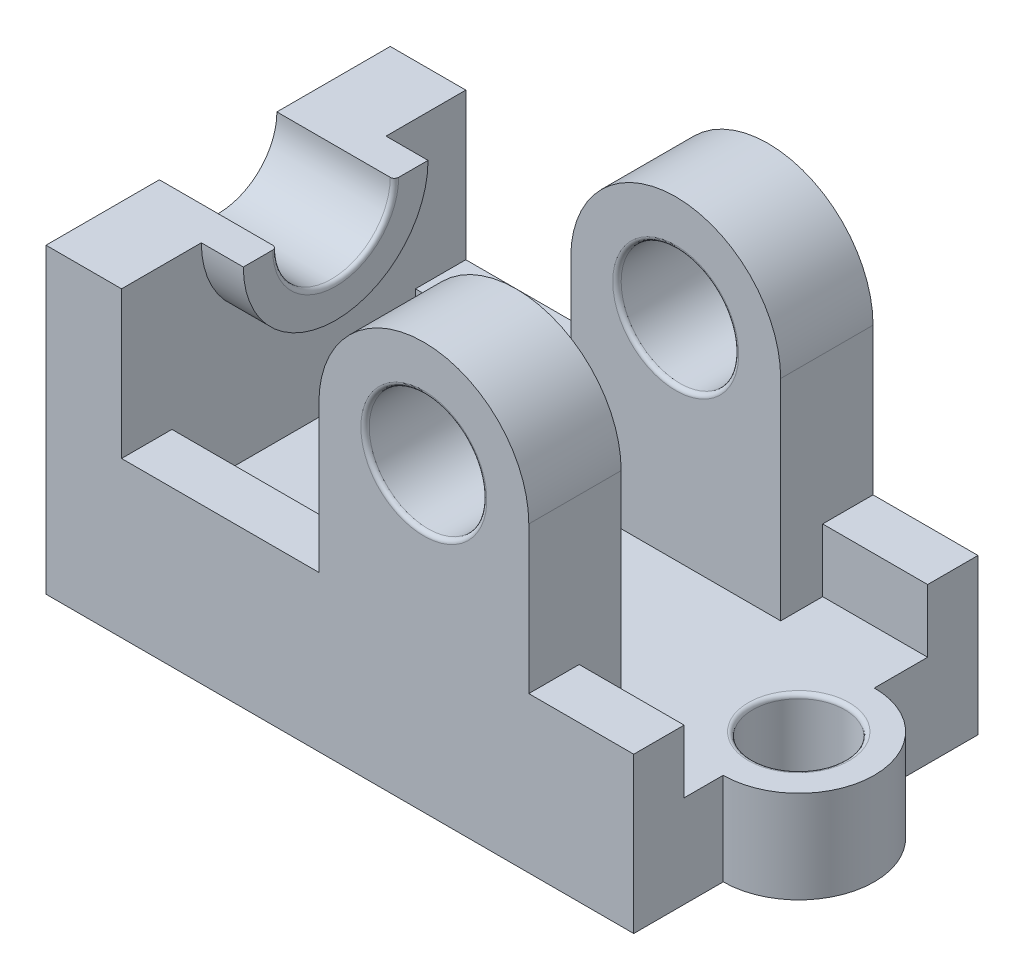
ISO-10303-21;
HEADER;
FILE_DESCRIPTION(('STEP AP214'),'2;1');
FILE_NAME('part.step','',(''),(''),'','','');
FILE_SCHEMA(('AUTOMOTIVE_DESIGN { 1 0 10303 214 1 1 1 1 }'));
ENDSEC;
DATA;
#1=APPLICATION_CONTEXT('core data for automotive mechanical design processes');
#2=APPLICATION_PROTOCOL_DEFINITION('international standard','automotive_design',2000,#1);
#3=PRODUCT_CONTEXT('',#1,'mechanical');
#4=PRODUCT('Part','Part','',(#3));
#5=PRODUCT_RELATED_PRODUCT_CATEGORY('part','',(#4));
#6=PRODUCT_DEFINITION_FORMATION('','',#4);
#7=PRODUCT_DEFINITION_CONTEXT('part definition',#1,'design');
#8=PRODUCT_DEFINITION('design','',#6,#7);
#9=PRODUCT_DEFINITION_SHAPE('','',#8);
#10=(LENGTH_UNIT() NAMED_UNIT(*) SI_UNIT(.MILLI.,.METRE.));
#11=(NAMED_UNIT(*) PLANE_ANGLE_UNIT() SI_UNIT($,.RADIAN.));
#12=(NAMED_UNIT(*) SI_UNIT($,.STERADIAN.) SOLID_ANGLE_UNIT());
#13=UNCERTAINTY_MEASURE_WITH_UNIT(LENGTH_MEASURE(1.E-05),#10,'distance_accuracy_value','');
#14=(GEOMETRIC_REPRESENTATION_CONTEXT(3) GLOBAL_UNCERTAINTY_ASSIGNED_CONTEXT((#13)) GLOBAL_UNIT_ASSIGNED_CONTEXT((#10,
#11,#12)) REPRESENTATION_CONTEXT('',''));
#15=CARTESIAN_POINT('',(0.,0.,0.));
#16=DIRECTION('',(0.,0.,1.));
#17=DIRECTION('',(1.,0.,0.));
#18=AXIS2_PLACEMENT_3D('',#15,#16,#17);
#19=CARTESIAN_POINT('',(0.,72.,0.));
#20=DIRECTION('',(0.,-1.,0.));
#21=DIRECTION('',(0.,0.,-1.));
#22=AXIS2_PLACEMENT_3D('',#19,#20,#21);
#23=PLANE('',#22);
#24=DIRECTION('',(0.,0.,1.));
#25=VECTOR('',#24,1.);
#26=CARTESIAN_POINT('',(-70.,72.,41.));
#27=LINE('',#26,#25);
#28=CARTESIAN_POINT('',(-70.,72.,-41.));
#29=VERTEX_POINT('',#28);
#30=CARTESIAN_POINT('',(-70.,72.,-14.));
#31=VERTEX_POINT('',#30);
#32=EDGE_CURVE('E270',#29,#31,#27,.T.);
#33=ORIENTED_EDGE('',*,*,#32,.T.);
#34=DIRECTION('',(-1.,0.,0.));
#35=VECTOR('',#34,1.);
#36=CARTESIAN_POINT('',(-42.,72.,-14.));
#37=LINE('',#36,#35);
#38=CARTESIAN_POINT('',(-43.,72.,-14.));
#39=VERTEX_POINT('',#38);
#40=EDGE_CURVE('E256',#39,#31,#37,.T.);
#41=ORIENTED_EDGE('',*,*,#40,.F.);
#42=CARTESIAN_POINT('',(-43.,72.,-15.));
#43=DIRECTION('',(0.,-1.,0.));
#44=DIRECTION('',(0.,0.,-1.));
#45=AXIS2_PLACEMENT_3D('',#42,#43,#44);
#46=CIRCLE('',#45,1.);
#47=CARTESIAN_POINT('',(-42.,72.,-15.));
#48=VERTEX_POINT('',#47);
#49=EDGE_CURVE('E63',#39,#48,#46,.F.);
#50=ORIENTED_EDGE('',*,*,#49,.T.);
#51=DIRECTION('',(0.,0.,-1.));
#52=VECTOR('',#51,1.);
#53=CARTESIAN_POINT('',(-42.,72.,-14.));
#54=LINE('',#53,#52);
#55=CARTESIAN_POINT('',(-42.,72.,-22.));
#56=VERTEX_POINT('',#55);
#57=EDGE_CURVE('E263',#48,#56,#54,.T.);
#58=ORIENTED_EDGE('',*,*,#57,.T.);
#59=DIRECTION('',(-1.,0.,0.));
#60=VECTOR('',#59,1.);
#61=CARTESIAN_POINT('',(-42.,72.,-22.));
#62=LINE('',#61,#60);
#63=CARTESIAN_POINT('',(-52.,72.,-22.));
#64=VERTEX_POINT('',#63);
#65=EDGE_CURVE('E544',#56,#64,#62,.T.);
#66=ORIENTED_EDGE('',*,*,#65,.T.);
#67=DIRECTION('',(0.,0.,-1.));
#68=VECTOR('',#67,1.);
#69=CARTESIAN_POINT('',(-52.,72.,-41.));
#70=LINE('',#69,#68);
#71=CARTESIAN_POINT('',(-52.,72.,-41.));
#72=VERTEX_POINT('',#71);
#73=EDGE_CURVE('E590',#64,#72,#70,.T.);
#74=ORIENTED_EDGE('',*,*,#73,.T.);
#75=DIRECTION('',(-1.,0.,0.));
#76=VECTOR('',#75,1.);
#77=CARTESIAN_POINT('',(-70.,72.,-41.));
#78=LINE('',#77,#76);
#79=EDGE_CURVE('E269',#72,#29,#78,.T.);
#80=ORIENTED_EDGE('',*,*,#79,.T.);
#81=EDGE_LOOP('',(#33,#41,#50,#58,#66,#74,#80));
#82=FACE_BOUND('',#81,.T.);
#83=ADVANCED_FACE('F47',(#82),#23,.F.);
#84=CARTESIAN_POINT('',(70.,22.,1.69184290030211));
#85=DIRECTION('',(0.,1.,0.));
#86=DIRECTION('',(0.,0.,1.));
#87=AXIS2_PLACEMENT_3D('',#84,#85,#86);
#88=PLANE('',#87);
#89=CARTESIAN_POINT('',(70.,22.,1.69184290030211));
#90=DIRECTION('',(0.,1.,0.));
#91=DIRECTION('',(0.,0.,1.));
#92=AXIS2_PLACEMENT_3D('',#89,#90,#91);
#93=CIRCLE('',#92,12.);
#94=CARTESIAN_POINT('',(70.,22.,13.6918429003021));
#95=VERTEX_POINT('',#94);
#96=EDGE_CURVE('E418',#95,#95,#93,.F.);
#97=ORIENTED_EDGE('',*,*,#96,.T.);
#98=EDGE_LOOP('',(#97));
#99=FACE_BOUND('',#98,.T.);
#100=DIRECTION('',(-1.,0.,0.));
#101=VECTOR('',#100,1.);
#102=CARTESIAN_POINT('',(0.,22.,-29.));
#103=LINE('',#102,#101);
#104=CARTESIAN_POINT('',(-4.99999999999997,22.,-29.));
#105=VERTEX_POINT('',#104);
#106=CARTESIAN_POINT('',(-52.,22.,-29.));
#107=VERTEX_POINT('',#106);
#108=EDGE_CURVE('E304',#105,#107,#103,.T.);
#109=ORIENTED_EDGE('',*,*,#108,.T.);
#110=DIRECTION('',(0.,0.,-1.));
#111=VECTOR('',#110,1.);
#112=CARTESIAN_POINT('',(-52.,22.,-41.));
#113=LINE('',#112,#111);
#114=CARTESIAN_POINT('',(-52.,22.,29.));
#115=VERTEX_POINT('',#114);
#116=EDGE_CURVE('E276',#115,#107,#113,.T.);
#117=ORIENTED_EDGE('',*,*,#116,.F.);
#118=DIRECTION('',(-1.,0.,0.));
#119=VECTOR('',#118,1.);
#120=CARTESIAN_POINT('',(0.,22.,29.));
#121=LINE('',#120,#119);
#122=CARTESIAN_POINT('',(-4.99999999999997,22.,29.));
#123=VERTEX_POINT('',#122);
#124=EDGE_CURVE('E328',#123,#115,#121,.T.);
#125=ORIENTED_EDGE('',*,*,#124,.F.);
#126=DIRECTION('',(0.,0.,1.));
#127=VECTOR('',#126,1.);
#128=CARTESIAN_POINT('',(-4.99999999999998,22.,19.));
#129=LINE('',#128,#127);
#130=CARTESIAN_POINT('',(-4.99999999999998,22.,19.));
#131=VERTEX_POINT('',#130);
#132=EDGE_CURVE('E577',#131,#123,#129,.T.);
#133=ORIENTED_EDGE('',*,*,#132,.F.);
#134=DIRECTION('',(-1.,0.,0.));
#135=VECTOR('',#134,1.);
#136=CARTESIAN_POINT('',(45.,22.,19.));
#137=LINE('',#136,#135);
#138=CARTESIAN_POINT('',(45.,22.,19.));
#139=VERTEX_POINT('',#138);
#140=EDGE_CURVE('E290',#139,#131,#137,.T.);
#141=ORIENTED_EDGE('',*,*,#140,.F.);
#142=DIRECTION('',(0.,0.,-1.));
#143=VECTOR('',#142,1.);
#144=CARTESIAN_POINT('',(45.,22.,41.));
#145=LINE('',#144,#143);
#146=CARTESIAN_POINT('',(45.,22.,29.));
#147=VERTEX_POINT('',#146);
#148=EDGE_CURVE('E573',#147,#139,#145,.T.);
#149=ORIENTED_EDGE('',*,*,#148,.F.);
#150=DIRECTION('',(-1.,0.,0.));
#151=VECTOR('',#150,1.);
#152=CARTESIAN_POINT('',(0.,22.,29.));
#153=LINE('',#152,#151);
#154=CARTESIAN_POINT('',(70.,22.,29.));
#155=VERTEX_POINT('',#154);
#156=EDGE_CURVE('E297',#155,#147,#153,.T.);
#157=ORIENTED_EDGE('',*,*,#156,.F.);
#158=DIRECTION('',(0.,0.,-1.));
#159=VECTOR('',#158,1.);
#160=CARTESIAN_POINT('',(70.,22.,41.));
#161=LINE('',#160,#159);
#162=CARTESIAN_POINT('',(70.,22.,19.6918429003021));
#163=VERTEX_POINT('',#162);
#164=EDGE_CURVE('E382',#155,#163,#161,.T.);
#165=ORIENTED_EDGE('',*,*,#164,.T.);
#166=CARTESIAN_POINT('',(70.,22.,1.69184290030211));
#167=DIRECTION('',(0.,1.,0.));
#168=DIRECTION('',(0.,0.,1.));
#169=AXIS2_PLACEMENT_3D('',#166,#167,#168);
#170=CIRCLE('',#169,18.);
#171=CARTESIAN_POINT('',(70.,22.,-16.3081570996979));
#172=VERTEX_POINT('',#171);
#173=EDGE_CURVE('E384',#163,#172,#170,.T.);
#174=ORIENTED_EDGE('',*,*,#173,.T.);
#175=DIRECTION('',(0.,0.,-1.));
#176=VECTOR('',#175,1.);
#177=CARTESIAN_POINT('',(70.,22.,-16.3081570996979));
#178=LINE('',#177,#176);
#179=CARTESIAN_POINT('',(70.,22.,-29.));
#180=VERTEX_POINT('',#179);
#181=EDGE_CURVE('E389',#172,#180,#178,.T.);
#182=ORIENTED_EDGE('',*,*,#181,.T.);
#183=DIRECTION('',(-1.,0.,0.));
#184=VECTOR('',#183,1.);
#185=CARTESIAN_POINT('',(0.,22.,-29.));
#186=LINE('',#185,#184);
#187=CARTESIAN_POINT('',(45.,22.,-29.));
#188=VERTEX_POINT('',#187);
#189=EDGE_CURVE('E321',#180,#188,#186,.T.);
#190=ORIENTED_EDGE('',*,*,#189,.T.);
#191=DIRECTION('',(0.,0.,-1.));
#192=VECTOR('',#191,1.);
#193=CARTESIAN_POINT('',(45.,22.,-19.));
#194=LINE('',#193,#192);
#195=CARTESIAN_POINT('',(45.,22.,-19.));
#196=VERTEX_POINT('',#195);
#197=EDGE_CURVE('E283',#196,#188,#194,.T.);
#198=ORIENTED_EDGE('',*,*,#197,.F.);
#199=DIRECTION('',(1.,0.,0.));
#200=VECTOR('',#199,1.);
#201=CARTESIAN_POINT('',(-4.99999999999997,22.,-19.));
#202=LINE('',#201,#200);
#203=CARTESIAN_POINT('',(-4.99999999999997,22.,-19.));
#204=VERTEX_POINT('',#203);
#205=EDGE_CURVE('E286',#204,#196,#202,.T.);
#206=ORIENTED_EDGE('',*,*,#205,.F.);
#207=DIRECTION('',(0.,0.,1.));
#208=VECTOR('',#207,1.);
#209=CARTESIAN_POINT('',(-4.99999999999997,22.,-41.));
#210=LINE('',#209,#208);
#211=EDGE_CURVE('E285',#105,#204,#210,.T.);
#212=ORIENTED_EDGE('',*,*,#211,.F.);
#213=EDGE_LOOP('',(#109,#117,#125,#133,#141,#149,#157,#165,#174,#182,#190,#198,#206,#212));
#214=FACE_BOUND('',#213,.T.);
#215=ADVANCED_FACE('F463',(#99,#214),#88,.T.);
#216=CARTESIAN_POINT('',(70.,0.,1.69184290030211));
#217=DIRECTION('',(0.,1.,0.));
#218=DIRECTION('',(0.,0.,1.));
#219=AXIS2_PLACEMENT_3D('',#216,#217,#218);
#220=PLANE('',#219);
#221=DIRECTION('',(-1.,0.,0.));
#222=VECTOR('',#221,1.);
#223=CARTESIAN_POINT('',(-70.,0.,-41.));
#224=LINE('',#223,#222);
#225=CARTESIAN_POINT('',(70.,0.,-41.));
#226=VERTEX_POINT('',#225);
#227=CARTESIAN_POINT('',(-70.,0.,-41.));
#228=VERTEX_POINT('',#227);
#229=EDGE_CURVE('E379',#226,#228,#224,.T.);
#230=ORIENTED_EDGE('',*,*,#229,.F.);
#231=DIRECTION('',(0.,0.,-1.));
#232=VECTOR('',#231,1.);
#233=CARTESIAN_POINT('',(70.,0.,-16.3081570996979));
#234=LINE('',#233,#232);
#235=CARTESIAN_POINT('',(70.,0.,-16.3081570996979));
#236=VERTEX_POINT('',#235);
#237=EDGE_CURVE('E381',#236,#226,#234,.T.);
#238=ORIENTED_EDGE('',*,*,#237,.F.);
#239=CARTESIAN_POINT('',(70.,0.,1.69184290030211));
#240=DIRECTION('',(0.,1.,0.));
#241=DIRECTION('',(0.,0.,1.));
#242=AXIS2_PLACEMENT_3D('',#239,#240,#241);
#243=CIRCLE('',#242,18.);
#244=CARTESIAN_POINT('',(70.,0.,19.6918429003021));
#245=VERTEX_POINT('',#244);
#246=EDGE_CURVE('E397',#245,#236,#243,.T.);
#247=ORIENTED_EDGE('',*,*,#246,.F.);
#248=DIRECTION('',(0.,0.,-1.));
#249=VECTOR('',#248,1.);
#250=CARTESIAN_POINT('',(70.,0.,41.));
#251=LINE('',#250,#249);
#252=CARTESIAN_POINT('',(70.,0.,41.));
#253=VERTEX_POINT('',#252);
#254=EDGE_CURVE('E396',#253,#245,#251,.T.);
#255=ORIENTED_EDGE('',*,*,#254,.F.);
#256=DIRECTION('',(1.,0.,0.));
#257=VECTOR('',#256,1.);
#258=CARTESIAN_POINT('',(-70.,0.,41.));
#259=LINE('',#258,#257);
#260=CARTESIAN_POINT('',(-70.,0.,41.));
#261=VERTEX_POINT('',#260);
#262=EDGE_CURVE('E395',#261,#253,#259,.T.);
#263=ORIENTED_EDGE('',*,*,#262,.F.);
#264=DIRECTION('',(0.,0.,1.));
#265=VECTOR('',#264,1.);
#266=CARTESIAN_POINT('',(-70.,0.,41.));
#267=LINE('',#266,#265);
#268=EDGE_CURVE('E394',#228,#261,#267,.T.);
#269=ORIENTED_EDGE('',*,*,#268,.F.);
#270=EDGE_LOOP('',(#230,#238,#247,#255,#263,#269));
#271=FACE_BOUND('',#270,.T.);
#272=CARTESIAN_POINT('',(70.,0.,1.69184290030211));
#273=DIRECTION('',(0.,1.,0.));
#274=DIRECTION('',(0.,0.,1.));
#275=AXIS2_PLACEMENT_3D('',#272,#273,#274);
#276=CIRCLE('',#275,11.);
#277=CARTESIAN_POINT('',(70.,0.,12.6918429003021));
#278=VERTEX_POINT('',#277);
#279=EDGE_CURVE('E380',#278,#278,#276,.T.);
#280=ORIENTED_EDGE('',*,*,#279,.T.);
#281=EDGE_LOOP('',(#280));
#282=FACE_BOUND('',#281,.T.);
#283=ADVANCED_FACE('F468',(#271,#282),#220,.F.);
#284=CARTESIAN_POINT('',(-70.,22.,-41.));
#285=DIRECTION('',(0.,0.,1.));
#286=DIRECTION('',(1.,0.,0.));
#287=AXIS2_PLACEMENT_3D('',#284,#285,#286);
#288=PLANE('',#287);
#289=CARTESIAN_POINT('',(20.,72.,-41.));
#290=DIRECTION('',(0.,0.,1.));
#291=DIRECTION('',(1.,0.,0.));
#292=AXIS2_PLACEMENT_3D('',#289,#290,#291);
#293=CIRCLE('',#292,15.);
#294=CARTESIAN_POINT('',(35.,72.,-41.));
#295=VERTEX_POINT('',#294);
#296=EDGE_CURVE('E11',#295,#295,#293,.T.);
#297=ORIENTED_EDGE('',*,*,#296,.T.);
#298=EDGE_LOOP('',(#297));
#299=FACE_BOUND('',#298,.T.);
#300=DIRECTION('',(0.,-1.,0.));
#301=VECTOR('',#300,1.);
#302=CARTESIAN_POINT('',(-4.99999999999997,72.,-41.));
#303=LINE('',#302,#301);
#304=CARTESIAN_POINT('',(-4.99999999999997,72.,-41.));
#305=VERTEX_POINT('',#304);
#306=CARTESIAN_POINT('',(-4.99999999999997,37.,-41.));
#307=VERTEX_POINT('',#306);
#308=EDGE_CURVE('E296',#305,#307,#303,.T.);
#309=ORIENTED_EDGE('',*,*,#308,.F.);
#310=CARTESIAN_POINT('',(20.,72.,-41.));
#311=DIRECTION('',(0.,0.,-1.));
#312=DIRECTION('',(-1.,0.,0.));
#313=AXIS2_PLACEMENT_3D('',#310,#311,#312);
#314=CIRCLE('',#313,25.);
#315=CARTESIAN_POINT('',(45.,72.,-41.));
#316=VERTEX_POINT('',#315);
#317=EDGE_CURVE('E553',#305,#316,#314,.T.);
#318=ORIENTED_EDGE('',*,*,#317,.T.);
#319=DIRECTION('',(0.,-1.,0.));
#320=VECTOR('',#319,1.);
#321=CARTESIAN_POINT('',(45.,72.,-41.));
#322=LINE('',#321,#320);
#323=CARTESIAN_POINT('',(45.,37.,-41.));
#324=VERTEX_POINT('',#323);
#325=EDGE_CURVE('E282',#316,#324,#322,.T.);
#326=ORIENTED_EDGE('',*,*,#325,.T.);
#327=DIRECTION('',(-1.,0.,0.));
#328=VECTOR('',#327,1.);
#329=CARTESIAN_POINT('',(0.,37.,-41.));
#330=LINE('',#329,#328);
#331=CARTESIAN_POINT('',(70.,37.,-41.));
#332=VERTEX_POINT('',#331);
#333=EDGE_CURVE('E370',#332,#324,#330,.T.);
#334=ORIENTED_EDGE('',*,*,#333,.F.);
#335=DIRECTION('',(0.,-1.,0.));
#336=VECTOR('',#335,1.);
#337=CARTESIAN_POINT('',(70.,22.,-41.));
#338=LINE('',#337,#336);
#339=EDGE_CURVE('E388',#332,#226,#338,.T.);
#340=ORIENTED_EDGE('',*,*,#339,.T.);
#341=ORIENTED_EDGE('',*,*,#229,.T.);
#342=DIRECTION('',(0.,-1.,0.));
#343=VECTOR('',#342,1.);
#344=CARTESIAN_POINT('',(-70.,22.,-41.));
#345=LINE('',#344,#343);
#346=EDGE_CURVE('E412',#29,#228,#345,.T.);
#347=ORIENTED_EDGE('',*,*,#346,.F.);
#348=ORIENTED_EDGE('',*,*,#79,.F.);
#349=DIRECTION('',(0.,-1.,0.));
#350=VECTOR('',#349,1.);
#351=CARTESIAN_POINT('',(-52.,72.,-41.));
#352=LINE('',#351,#350);
#353=CARTESIAN_POINT('',(-52.,37.,-41.));
#354=VERTEX_POINT('',#353);
#355=EDGE_CURVE('E588',#72,#354,#352,.T.);
#356=ORIENTED_EDGE('',*,*,#355,.T.);
#357=DIRECTION('',(-1.,0.,0.));
#358=VECTOR('',#357,1.);
#359=CARTESIAN_POINT('',(0.,37.,-41.));
#360=LINE('',#359,#358);
#361=EDGE_CURVE('E308',#307,#354,#360,.T.);
#362=ORIENTED_EDGE('',*,*,#361,.F.);
#363=EDGE_LOOP('',(#309,#318,#326,#334,#340,#341,#347,#348,#356,#362));
#364=FACE_BOUND('',#363,.T.);
#365=ADVANCED_FACE('F596',(#299,#364),#288,.F.);
#366=CARTESIAN_POINT('',(-70.,22.,41.));
#367=DIRECTION('',(1.,0.,0.));
#368=DIRECTION('',(0.,0.,-1.));
#369=AXIS2_PLACEMENT_3D('',#366,#367,#368);
#370=PLANE('',#369);
#371=CARTESIAN_POINT('',(-70.,72.,14.));
#372=VERTEX_POINT('',#371);
#373=CARTESIAN_POINT('',(-70.,72.,41.));
#374=VERTEX_POINT('',#373);
#375=EDGE_CURVE('E242',#372,#374,#27,.T.);
#376=ORIENTED_EDGE('',*,*,#375,.F.);
#377=CARTESIAN_POINT('',(-70.,72.,0.));
#378=DIRECTION('',(1.,0.,0.));
#379=DIRECTION('',(0.,0.,-1.));
#380=AXIS2_PLACEMENT_3D('',#377,#378,#379);
#381=CIRCLE('',#380,14.);
#382=EDGE_CURVE('E253',#372,#31,#381,.T.);
#383=ORIENTED_EDGE('',*,*,#382,.T.);
#384=ORIENTED_EDGE('',*,*,#32,.F.);
#385=ORIENTED_EDGE('',*,*,#346,.T.);
#386=ORIENTED_EDGE('',*,*,#268,.T.);
#387=DIRECTION('',(0.,-1.,0.));
#388=VECTOR('',#387,1.);
#389=CARTESIAN_POINT('',(-70.,22.,41.));
#390=LINE('',#389,#388);
#391=EDGE_CURVE('E261',#374,#261,#390,.T.);
#392=ORIENTED_EDGE('',*,*,#391,.F.);
#393=EDGE_LOOP('',(#376,#383,#384,#385,#386,#392));
#394=FACE_BOUND('',#393,.T.);
#395=ADVANCED_FACE('F262',(#394),#370,.F.);
#396=CARTESIAN_POINT('',(-70.,22.,41.));
#397=DIRECTION('',(0.,0.,-1.));
#398=DIRECTION('',(-1.,0.,0.));
#399=AXIS2_PLACEMENT_3D('',#396,#397,#398);
#400=PLANE('',#399);
#401=CARTESIAN_POINT('',(20.,72.,41.));
#402=DIRECTION('',(0.,0.,-1.));
#403=DIRECTION('',(-1.,0.,0.));
#404=AXIS2_PLACEMENT_3D('',#401,#402,#403);
#405=CIRCLE('',#404,15.);
#406=CARTESIAN_POINT('',(5.00000000000003,72.,41.));
#407=VERTEX_POINT('',#406);
#408=EDGE_CURVE('E445',#407,#407,#405,.T.);
#409=ORIENTED_EDGE('',*,*,#408,.T.);
#410=EDGE_LOOP('',(#409));
#411=FACE_BOUND('',#410,.T.);
#412=ORIENTED_EDGE('',*,*,#262,.T.);
#413=DIRECTION('',(0.,-1.,0.));
#414=VECTOR('',#413,1.);
#415=CARTESIAN_POINT('',(70.,22.,41.));
#416=LINE('',#415,#414);
#417=CARTESIAN_POINT('',(70.,37.,41.));
#418=VERTEX_POINT('',#417);
#419=EDGE_CURVE('E408',#418,#253,#416,.T.);
#420=ORIENTED_EDGE('',*,*,#419,.F.);
#421=DIRECTION('',(1.,0.,0.));
#422=VECTOR('',#421,1.);
#423=CARTESIAN_POINT('',(0.,37.,41.));
#424=LINE('',#423,#422);
#425=CARTESIAN_POINT('',(45.,37.,41.));
#426=VERTEX_POINT('',#425);
#427=EDGE_CURVE('E347',#426,#418,#424,.T.);
#428=ORIENTED_EDGE('',*,*,#427,.F.);
#429=DIRECTION('',(0.,-1.,0.));
#430=VECTOR('',#429,1.);
#431=CARTESIAN_POINT('',(45.,72.,41.));
#432=LINE('',#431,#430);
#433=CARTESIAN_POINT('',(45.,72.,41.));
#434=VERTEX_POINT('',#433);
#435=EDGE_CURVE('E568',#434,#426,#432,.T.);
#436=ORIENTED_EDGE('',*,*,#435,.F.);
#437=CARTESIAN_POINT('',(20.,72.,41.));
#438=DIRECTION('',(0.,0.,1.));
#439=DIRECTION('',(1.,0.,0.));
#440=AXIS2_PLACEMENT_3D('',#437,#438,#439);
#441=CIRCLE('',#440,25.);
#442=CARTESIAN_POINT('',(-4.99999999999997,72.,41.));
#443=VERTEX_POINT('',#442);
#444=EDGE_CURVE('E555',#434,#443,#441,.T.);
#445=ORIENTED_EDGE('',*,*,#444,.T.);
#446=DIRECTION('',(0.,-1.,0.));
#447=VECTOR('',#446,1.);
#448=CARTESIAN_POINT('',(-4.99999999999997,72.,41.));
#449=LINE('',#448,#447);
#450=CARTESIAN_POINT('',(-4.99999999999997,37.,41.));
#451=VERTEX_POINT('',#450);
#452=EDGE_CURVE('E564',#443,#451,#449,.T.);
#453=ORIENTED_EDGE('',*,*,#452,.T.);
#454=DIRECTION('',(1.,0.,0.));
#455=VECTOR('',#454,1.);
#456=CARTESIAN_POINT('',(0.,37.,41.));
#457=LINE('',#456,#455);
#458=CARTESIAN_POINT('',(-52.,37.,41.));
#459=VERTEX_POINT('',#458);
#460=EDGE_CURVE('E335',#459,#451,#457,.T.);
#461=ORIENTED_EDGE('',*,*,#460,.F.);
#462=DIRECTION('',(0.,-1.,0.));
#463=VECTOR('',#462,1.);
#464=CARTESIAN_POINT('',(-52.,72.,41.));
#465=LINE('',#464,#463);
#466=CARTESIAN_POINT('',(-52.,72.,41.));
#467=VERTEX_POINT('',#466);
#468=EDGE_CURVE('E557',#467,#459,#465,.T.);
#469=ORIENTED_EDGE('',*,*,#468,.F.);
#470=DIRECTION('',(1.,0.,0.));
#471=VECTOR('',#470,1.);
#472=CARTESIAN_POINT('',(-52.,72.,41.));
#473=LINE('',#472,#471);
#474=EDGE_CURVE('E267',#374,#467,#473,.T.);
#475=ORIENTED_EDGE('',*,*,#474,.F.);
#476=ORIENTED_EDGE('',*,*,#391,.T.);
#477=EDGE_LOOP('',(#412,#420,#428,#436,#445,#453,#461,#469,#475,#476));
#478=FACE_BOUND('',#477,.T.);
#479=ADVANCED_FACE('F605',(#411,#478),#400,.F.);
#480=CARTESIAN_POINT('',(70.,22.,41.));
#481=DIRECTION('',(-1.,0.,0.));
#482=DIRECTION('',(0.,0.,1.));
#483=AXIS2_PLACEMENT_3D('',#480,#481,#482);
#484=PLANE('',#483);
#485=ORIENTED_EDGE('',*,*,#254,.T.);
#486=DIRECTION('',(0.,-1.,0.));
#487=VECTOR('',#486,1.);
#488=CARTESIAN_POINT('',(70.,22.,19.6918429003021));
#489=LINE('',#488,#487);
#490=EDGE_CURVE('E409',#163,#245,#489,.T.);
#491=ORIENTED_EDGE('',*,*,#490,.F.);
#492=ORIENTED_EDGE('',*,*,#164,.F.);
#493=DIRECTION('',(0.,-1.,0.));
#494=VECTOR('',#493,1.);
#495=CARTESIAN_POINT('',(70.,37.,29.));
#496=LINE('',#495,#494);
#497=CARTESIAN_POINT('',(70.,37.,29.));
#498=VERTEX_POINT('',#497);
#499=EDGE_CURVE('E352',#498,#155,#496,.T.);
#500=ORIENTED_EDGE('',*,*,#499,.F.);
#501=DIRECTION('',(0.,0.,-1.));
#502=VECTOR('',#501,1.);
#503=CARTESIAN_POINT('',(70.,37.,0.));
#504=LINE('',#503,#502);
#505=EDGE_CURVE('E351',#418,#498,#504,.T.);
#506=ORIENTED_EDGE('',*,*,#505,.F.);
#507=ORIENTED_EDGE('',*,*,#419,.T.);
#508=EDGE_LOOP('',(#485,#491,#492,#500,#506,#507));
#509=FACE_BOUND('',#508,.T.);
#510=ADVANCED_FACE('F611',(#509),#484,.F.);
#511=CARTESIAN_POINT('',(70.,22.,1.69184290030211));
#512=DIRECTION('',(0.,-1.,0.));
#513=DIRECTION('',(0.,0.,-1.));
#514=AXIS2_PLACEMENT_3D('',#511,#512,#513);
#515=CYLINDRICAL_SURFACE('',#514,18.);
#516=ORIENTED_EDGE('',*,*,#246,.T.);
#517=DIRECTION('',(0.,-1.,0.));
#518=VECTOR('',#517,1.);
#519=CARTESIAN_POINT('',(70.,22.,-16.3081570996979));
#520=LINE('',#519,#518);
#521=EDGE_CURVE('E401',#172,#236,#520,.T.);
#522=ORIENTED_EDGE('',*,*,#521,.F.);
#523=ORIENTED_EDGE('',*,*,#173,.F.);
#524=ORIENTED_EDGE('',*,*,#490,.T.);
#525=EDGE_LOOP('',(#516,#522,#523,#524));
#526=FACE_BOUND('',#525,.T.);
#527=ADVANCED_FACE('F618',(#526),#515,.T.);
#528=CARTESIAN_POINT('',(70.,22.,-16.3081570996979));
#529=DIRECTION('',(-1.,0.,0.));
#530=DIRECTION('',(0.,0.,1.));
#531=AXIS2_PLACEMENT_3D('',#528,#529,#530);
#532=PLANE('',#531);
#533=ORIENTED_EDGE('',*,*,#237,.T.);
#534=ORIENTED_EDGE('',*,*,#339,.F.);
#535=DIRECTION('',(0.,0.,-1.));
#536=VECTOR('',#535,1.);
#537=CARTESIAN_POINT('',(70.,37.,0.));
#538=LINE('',#537,#536);
#539=CARTESIAN_POINT('',(70.,37.,-29.));
#540=VERTEX_POINT('',#539);
#541=EDGE_CURVE('E364',#540,#332,#538,.T.);
#542=ORIENTED_EDGE('',*,*,#541,.F.);
#543=DIRECTION('',(0.,-1.,0.));
#544=VECTOR('',#543,1.);
#545=CARTESIAN_POINT('',(70.,37.,-29.));
#546=LINE('',#545,#544);
#547=EDGE_CURVE('E369',#540,#180,#546,.T.);
#548=ORIENTED_EDGE('',*,*,#547,.T.);
#549=ORIENTED_EDGE('',*,*,#181,.F.);
#550=ORIENTED_EDGE('',*,*,#521,.T.);
#551=EDGE_LOOP('',(#533,#534,#542,#548,#549,#550));
#552=FACE_BOUND('',#551,.T.);
#553=ADVANCED_FACE('F667',(#552),#532,.F.);
#554=CARTESIAN_POINT('',(70.,22.,1.69184290030211));
#555=DIRECTION('',(0.,-1.,0.));
#556=DIRECTION('',(0.,0.,-1.));
#557=AXIS2_PLACEMENT_3D('',#554,#555,#556);
#558=CYLINDRICAL_SURFACE('',#557,11.);
#559=CARTESIAN_POINT('',(70.,21.,1.69184290030211));
#560=DIRECTION('',(0.,1.,0.));
#561=DIRECTION('',(0.,0.,1.));
#562=AXIS2_PLACEMENT_3D('',#559,#560,#561);
#563=CIRCLE('',#562,11.);
#564=CARTESIAN_POINT('',(70.,21.,12.6918429003021));
#565=VERTEX_POINT('',#564);
#566=EDGE_CURVE('E416',#565,#565,#563,.T.);
#567=ORIENTED_EDGE('',*,*,#566,.T.);
#568=EDGE_LOOP('',(#567));
#569=FACE_BOUND('',#568,.T.);
#570=ORIENTED_EDGE('',*,*,#279,.F.);
#571=EDGE_LOOP('',(#570));
#572=FACE_BOUND('',#571,.T.);
#573=ADVANCED_FACE('F671',(#569,#572),#558,.F.);
#574=CARTESIAN_POINT('',(0.,37.,-29.));
#575=DIRECTION('',(0.,0.,1.));
#576=DIRECTION('',(1.,0.,0.));
#577=AXIS2_PLACEMENT_3D('',#574,#575,#576);
#578=PLANE('',#577);
#579=ORIENTED_EDGE('',*,*,#189,.F.);
#580=ORIENTED_EDGE('',*,*,#547,.F.);
#581=DIRECTION('',(-1.,0.,0.));
#582=VECTOR('',#581,1.);
#583=CARTESIAN_POINT('',(0.,37.,-29.));
#584=LINE('',#583,#582);
#585=CARTESIAN_POINT('',(45.,37.,-29.));
#586=VERTEX_POINT('',#585);
#587=EDGE_CURVE('E363',#540,#586,#584,.T.);
#588=ORIENTED_EDGE('',*,*,#587,.T.);
#589=DIRECTION('',(0.,-1.,0.));
#590=VECTOR('',#589,1.);
#591=CARTESIAN_POINT('',(45.,37.,-29.));
#592=LINE('',#591,#590);
#593=EDGE_CURVE('E372',#586,#188,#592,.T.);
#594=ORIENTED_EDGE('',*,*,#593,.T.);
#595=EDGE_LOOP('',(#579,#580,#588,#594));
#596=FACE_BOUND('',#595,.T.);
#597=ADVANCED_FACE('F672',(#596),#578,.T.);
#598=CARTESIAN_POINT('',(0.,37.,0.));
#599=DIRECTION('',(0.,1.,0.));
#600=DIRECTION('',(0.,0.,1.));
#601=AXIS2_PLACEMENT_3D('',#598,#599,#600);
#602=PLANE('',#601);
#603=DIRECTION('',(0.,0.,-1.));
#604=VECTOR('',#603,1.);
#605=CARTESIAN_POINT('',(45.,37.,0.));
#606=LINE('',#605,#604);
#607=EDGE_CURVE('E360',#586,#324,#606,.T.);
#608=ORIENTED_EDGE('',*,*,#607,.F.);
#609=ORIENTED_EDGE('',*,*,#587,.F.);
#610=ORIENTED_EDGE('',*,*,#541,.T.);
#611=ORIENTED_EDGE('',*,*,#333,.T.);
#612=EDGE_LOOP('',(#608,#609,#610,#611));
#613=FACE_BOUND('',#612,.T.);
#614=ADVANCED_FACE('F669',(#613),#602,.T.);
#615=CARTESIAN_POINT('',(0.,37.,-29.));
#616=DIRECTION('',(0.,0.,1.));
#617=DIRECTION('',(1.,0.,0.));
#618=AXIS2_PLACEMENT_3D('',#615,#616,#617);
#619=PLANE('',#618);
#620=ORIENTED_EDGE('',*,*,#108,.F.);
#621=DIRECTION('',(0.,-1.,0.));
#622=VECTOR('',#621,1.);
#623=CARTESIAN_POINT('',(-4.99999999999997,37.,-29.));
#624=LINE('',#623,#622);
#625=CARTESIAN_POINT('',(-4.99999999999997,37.,-29.));
#626=VERTEX_POINT('',#625);
#627=EDGE_CURVE('E318',#626,#105,#624,.T.);
#628=ORIENTED_EDGE('',*,*,#627,.F.);
#629=DIRECTION('',(-1.,0.,0.));
#630=VECTOR('',#629,1.);
#631=CARTESIAN_POINT('',(0.,37.,-29.));
#632=LINE('',#631,#630);
#633=CARTESIAN_POINT('',(-52.,37.,-29.));
#634=VERTEX_POINT('',#633);
#635=EDGE_CURVE('E301',#626,#634,#632,.T.);
#636=ORIENTED_EDGE('',*,*,#635,.T.);
#637=DIRECTION('',(0.,-1.,0.));
#638=VECTOR('',#637,1.);
#639=CARTESIAN_POINT('',(-52.,37.,-29.));
#640=LINE('',#639,#638);
#641=EDGE_CURVE('E313',#634,#107,#640,.T.);
#642=ORIENTED_EDGE('',*,*,#641,.T.);
#643=EDGE_LOOP('',(#620,#628,#636,#642));
#644=FACE_BOUND('',#643,.T.);
#645=ADVANCED_FACE('F647',(#644),#619,.T.);
#646=CARTESIAN_POINT('',(0.,37.,0.));
#647=DIRECTION('',(0.,1.,0.));
#648=DIRECTION('',(0.,0.,1.));
#649=AXIS2_PLACEMENT_3D('',#646,#647,#648);
#650=PLANE('',#649);
#651=ORIENTED_EDGE('',*,*,#635,.F.);
#652=DIRECTION('',(0.,0.,-1.));
#653=VECTOR('',#652,1.);
#654=CARTESIAN_POINT('',(-4.99999999999997,37.,0.));
#655=LINE('',#654,#653);
#656=EDGE_CURVE('E302',#626,#307,#655,.T.);
#657=ORIENTED_EDGE('',*,*,#656,.T.);
#658=ORIENTED_EDGE('',*,*,#361,.T.);
#659=DIRECTION('',(0.,0.,1.));
#660=VECTOR('',#659,1.);
#661=CARTESIAN_POINT('',(-52.,37.,0.));
#662=LINE('',#661,#660);
#663=EDGE_CURVE('E311',#354,#634,#662,.T.);
#664=ORIENTED_EDGE('',*,*,#663,.T.);
#665=EDGE_LOOP('',(#651,#657,#658,#664));
#666=FACE_BOUND('',#665,.T.);
#667=ADVANCED_FACE('F652',(#666),#650,.T.);
#668=CARTESIAN_POINT('',(0.,37.,29.));
#669=DIRECTION('',(0.,0.,1.));
#670=DIRECTION('',(1.,0.,0.));
#671=AXIS2_PLACEMENT_3D('',#668,#669,#670);
#672=PLANE('',#671);
#673=ORIENTED_EDGE('',*,*,#124,.T.);
#674=DIRECTION('',(0.,-1.,0.));
#675=VECTOR('',#674,1.);
#676=CARTESIAN_POINT('',(-52.,37.,29.));
#677=LINE('',#676,#675);
#678=CARTESIAN_POINT('',(-52.,37.,29.));
#679=VERTEX_POINT('',#678);
#680=EDGE_CURVE('E334',#679,#115,#677,.T.);
#681=ORIENTED_EDGE('',*,*,#680,.F.);
#682=DIRECTION('',(-1.,0.,0.));
#683=VECTOR('',#682,1.);
#684=CARTESIAN_POINT('',(0.,37.,29.));
#685=LINE('',#684,#683);
#686=CARTESIAN_POINT('',(-4.99999999999997,37.,29.));
#687=VERTEX_POINT('',#686);
#688=EDGE_CURVE('E322',#687,#679,#685,.T.);
#689=ORIENTED_EDGE('',*,*,#688,.F.);
#690=DIRECTION('',(0.,-1.,0.));
#691=VECTOR('',#690,1.);
#692=CARTESIAN_POINT('',(-4.99999999999997,37.,29.));
#693=LINE('',#692,#691);
#694=EDGE_CURVE('E320',#687,#123,#693,.T.);
#695=ORIENTED_EDGE('',*,*,#694,.T.);
#696=EDGE_LOOP('',(#673,#681,#689,#695));
#697=FACE_BOUND('',#696,.T.);
#698=ADVANCED_FACE('F639',(#697),#672,.F.);
#699=CARTESIAN_POINT('',(0.,37.,0.));
#700=DIRECTION('',(0.,1.,0.));
#701=DIRECTION('',(0.,0.,1.));
#702=AXIS2_PLACEMENT_3D('',#699,#700,#701);
#703=PLANE('',#702);
#704=DIRECTION('',(0.,0.,1.));
#705=VECTOR('',#704,1.);
#706=CARTESIAN_POINT('',(-4.99999999999996,37.,0.));
#707=LINE('',#706,#705);
#708=EDGE_CURVE('E325',#687,#451,#707,.T.);
#709=ORIENTED_EDGE('',*,*,#708,.F.);
#710=ORIENTED_EDGE('',*,*,#688,.T.);
#711=DIRECTION('',(0.,0.,1.));
#712=VECTOR('',#711,1.);
#713=CARTESIAN_POINT('',(-52.,37.,0.));
#714=LINE('',#713,#712);
#715=EDGE_CURVE('E330',#679,#459,#714,.T.);
#716=ORIENTED_EDGE('',*,*,#715,.T.);
#717=ORIENTED_EDGE('',*,*,#460,.T.);
#718=EDGE_LOOP('',(#709,#710,#716,#717));
#719=FACE_BOUND('',#718,.T.);
#720=ADVANCED_FACE('F645',(#719),#703,.T.);
#721=CARTESIAN_POINT('',(0.,37.,29.));
#722=DIRECTION('',(0.,0.,1.));
#723=DIRECTION('',(1.,0.,0.));
#724=AXIS2_PLACEMENT_3D('',#721,#722,#723);
#725=PLANE('',#724);
#726=ORIENTED_EDGE('',*,*,#156,.T.);
#727=DIRECTION('',(0.,-1.,0.));
#728=VECTOR('',#727,1.);
#729=CARTESIAN_POINT('',(45.,37.,29.));
#730=LINE('',#729,#728);
#731=CARTESIAN_POINT('',(45.,37.,29.));
#732=VERTEX_POINT('',#731);
#733=EDGE_CURVE('E336',#732,#147,#730,.T.);
#734=ORIENTED_EDGE('',*,*,#733,.F.);
#735=DIRECTION('',(-1.,0.,0.));
#736=VECTOR('',#735,1.);
#737=CARTESIAN_POINT('',(0.,37.,29.));
#738=LINE('',#737,#736);
#739=EDGE_CURVE('E341',#498,#732,#738,.T.);
#740=ORIENTED_EDGE('',*,*,#739,.F.);
#741=ORIENTED_EDGE('',*,*,#499,.T.);
#742=EDGE_LOOP('',(#726,#734,#740,#741));
#743=FACE_BOUND('',#742,.T.);
#744=ADVANCED_FACE('F624',(#743),#725,.F.);
#745=CARTESIAN_POINT('',(0.,37.,0.));
#746=DIRECTION('',(0.,1.,0.));
#747=DIRECTION('',(0.,0.,1.));
#748=AXIS2_PLACEMENT_3D('',#745,#746,#747);
#749=PLANE('',#748);
#750=ORIENTED_EDGE('',*,*,#739,.T.);
#751=DIRECTION('',(0.,0.,1.));
#752=VECTOR('',#751,1.);
#753=CARTESIAN_POINT('',(45.,37.,0.));
#754=LINE('',#753,#752);
#755=EDGE_CURVE('E342',#732,#426,#754,.T.);
#756=ORIENTED_EDGE('',*,*,#755,.T.);
#757=ORIENTED_EDGE('',*,*,#427,.T.);
#758=ORIENTED_EDGE('',*,*,#505,.T.);
#759=EDGE_LOOP('',(#750,#756,#757,#758));
#760=FACE_BOUND('',#759,.T.);
#761=ADVANCED_FACE('F501',(#760),#749,.T.);
#762=CARTESIAN_POINT('',(-4.99999999999998,72.,19.));
#763=DIRECTION('',(1.,0.,0.));
#764=DIRECTION('',(0.,0.,-1.));
#765=AXIS2_PLACEMENT_3D('',#762,#763,#764);
#766=PLANE('',#765);
#767=ORIENTED_EDGE('',*,*,#132,.T.);
#768=ORIENTED_EDGE('',*,*,#694,.F.);
#769=ORIENTED_EDGE('',*,*,#708,.T.);
#770=ORIENTED_EDGE('',*,*,#452,.F.);
#771=DIRECTION('',(0.,0.,1.));
#772=VECTOR('',#771,1.);
#773=CARTESIAN_POINT('',(-4.99999999999998,72.,19.));
#774=LINE('',#773,#772);
#775=CARTESIAN_POINT('',(-4.99999999999998,72.,19.));
#776=VERTEX_POINT('',#775);
#777=EDGE_CURVE('E580',#776,#443,#774,.T.);
#778=ORIENTED_EDGE('',*,*,#777,.F.);
#779=DIRECTION('',(0.,-1.,0.));
#780=VECTOR('',#779,1.);
#781=CARTESIAN_POINT('',(-4.99999999999998,72.,19.));
#782=LINE('',#781,#780);
#783=EDGE_CURVE('E563',#776,#131,#782,.T.);
#784=ORIENTED_EDGE('',*,*,#783,.T.);
#785=EDGE_LOOP('',(#767,#768,#769,#770,#778,#784));
#786=FACE_BOUND('',#785,.T.);
#787=ADVANCED_FACE('F498',(#786),#766,.F.);
#788=CARTESIAN_POINT('',(45.,72.,41.));
#789=DIRECTION('',(-1.,0.,0.));
#790=DIRECTION('',(0.,0.,1.));
#791=AXIS2_PLACEMENT_3D('',#788,#789,#790);
#792=PLANE('',#791);
#793=ORIENTED_EDGE('',*,*,#755,.F.);
#794=ORIENTED_EDGE('',*,*,#733,.T.);
#795=ORIENTED_EDGE('',*,*,#148,.T.);
#796=DIRECTION('',(0.,-1.,0.));
#797=VECTOR('',#796,1.);
#798=CARTESIAN_POINT('',(45.,72.,19.));
#799=LINE('',#798,#797);
#800=CARTESIAN_POINT('',(45.,72.,19.));
#801=VERTEX_POINT('',#800);
#802=EDGE_CURVE('E569',#801,#139,#799,.T.);
#803=ORIENTED_EDGE('',*,*,#802,.F.);
#804=DIRECTION('',(0.,0.,-1.));
#805=VECTOR('',#804,1.);
#806=CARTESIAN_POINT('',(45.,72.,41.));
#807=LINE('',#806,#805);
#808=EDGE_CURVE('E572',#434,#801,#807,.T.);
#809=ORIENTED_EDGE('',*,*,#808,.F.);
#810=ORIENTED_EDGE('',*,*,#435,.T.);
#811=EDGE_LOOP('',(#793,#794,#795,#803,#809,#810));
#812=FACE_BOUND('',#811,.T.);
#813=ADVANCED_FACE('F495',(#812),#792,.F.);
#814=CARTESIAN_POINT('',(45.,72.,19.));
#815=DIRECTION('',(0.,0.,1.));
#816=DIRECTION('',(1.,0.,0.));
#817=AXIS2_PLACEMENT_3D('',#814,#815,#816);
#818=PLANE('',#817);
#819=CARTESIAN_POINT('',(20.,72.,19.));
#820=DIRECTION('',(0.,0.,1.));
#821=DIRECTION('',(1.,0.,0.));
#822=AXIS2_PLACEMENT_3D('',#819,#820,#821);
#823=CIRCLE('',#822,15.);
#824=CARTESIAN_POINT('',(35.,72.,19.));
#825=VERTEX_POINT('',#824);
#826=EDGE_CURVE('E60',#825,#825,#823,.T.);
#827=ORIENTED_EDGE('',*,*,#826,.T.);
#828=EDGE_LOOP('',(#827));
#829=FACE_BOUND('',#828,.T.);
#830=ORIENTED_EDGE('',*,*,#783,.F.);
#831=CARTESIAN_POINT('',(20.,72.,19.));
#832=DIRECTION('',(0.,0.,1.));
#833=DIRECTION('',(1.,0.,0.));
#834=AXIS2_PLACEMENT_3D('',#831,#832,#833);
#835=CIRCLE('',#834,25.);
#836=EDGE_CURVE('E560',#801,#776,#835,.T.);
#837=ORIENTED_EDGE('',*,*,#836,.F.);
#838=ORIENTED_EDGE('',*,*,#802,.T.);
#839=ORIENTED_EDGE('',*,*,#140,.T.);
#840=EDGE_LOOP('',(#830,#837,#838,#839));
#841=FACE_BOUND('',#840,.T.);
#842=ADVANCED_FACE('F450',(#829,#841),#818,.F.);
#843=CARTESIAN_POINT('',(-52.,72.,-41.));
#844=DIRECTION('',(-1.,0.,0.));
#845=DIRECTION('',(0.,0.,1.));
#846=AXIS2_PLACEMENT_3D('',#843,#844,#845);
#847=PLANE('',#846);
#848=ORIENTED_EDGE('',*,*,#73,.F.);
#849=CARTESIAN_POINT('',(-52.,72.,0.));
#850=DIRECTION('',(-1.,0.,0.));
#851=DIRECTION('',(0.,0.,1.));
#852=AXIS2_PLACEMENT_3D('',#849,#850,#851);
#853=CIRCLE('',#852,22.);
#854=CARTESIAN_POINT('',(-52.,72.,22.));
#855=VERTEX_POINT('',#854);
#856=EDGE_CURVE('E252',#64,#855,#853,.T.);
#857=ORIENTED_EDGE('',*,*,#856,.T.);
#858=EDGE_CURVE('E272',#467,#855,#70,.T.);
#859=ORIENTED_EDGE('',*,*,#858,.F.);
#860=ORIENTED_EDGE('',*,*,#468,.T.);
#861=ORIENTED_EDGE('',*,*,#715,.F.);
#862=ORIENTED_EDGE('',*,*,#680,.T.);
#863=ORIENTED_EDGE('',*,*,#116,.T.);
#864=ORIENTED_EDGE('',*,*,#641,.F.);
#865=ORIENTED_EDGE('',*,*,#663,.F.);
#866=ORIENTED_EDGE('',*,*,#355,.F.);
#867=EDGE_LOOP('',(#848,#857,#859,#860,#861,#862,#863,#864,#865,#866));
#868=FACE_BOUND('',#867,.T.);
#869=ADVANCED_FACE('F479',(#868),#847,.F.);
#870=DIRECTION('',(-1.,0.,0.));
#871=VECTOR('',#870,1.);
#872=CARTESIAN_POINT('',(-42.,72.,14.));
#873=LINE('',#872,#871);
#874=CARTESIAN_POINT('',(-43.,72.,14.));
#875=VERTEX_POINT('',#874);
#876=EDGE_CURVE('E239',#875,#372,#873,.T.);
#877=ORIENTED_EDGE('',*,*,#876,.T.);
#878=ORIENTED_EDGE('',*,*,#375,.T.);
#879=ORIENTED_EDGE('',*,*,#474,.T.);
#880=ORIENTED_EDGE('',*,*,#858,.T.);
#881=DIRECTION('',(-1.,0.,0.));
#882=VECTOR('',#881,1.);
#883=CARTESIAN_POINT('',(-42.,72.,22.));
#884=LINE('',#883,#882);
#885=CARTESIAN_POINT('',(-42.,72.,22.));
#886=VERTEX_POINT('',#885);
#887=EDGE_CURVE('E255',#886,#855,#884,.T.);
#888=ORIENTED_EDGE('',*,*,#887,.F.);
#889=DIRECTION('',(0.,0.,-1.));
#890=VECTOR('',#889,1.);
#891=CARTESIAN_POINT('',(-42.,72.,14.));
#892=LINE('',#891,#890);
#893=CARTESIAN_POINT('',(-42.,72.,15.));
#894=VERTEX_POINT('',#893);
#895=EDGE_CURVE('E542',#886,#894,#892,.T.);
#896=ORIENTED_EDGE('',*,*,#895,.T.);
#897=CARTESIAN_POINT('',(-43.,72.,15.));
#898=DIRECTION('',(0.,-1.,0.));
#899=DIRECTION('',(0.,0.,-1.));
#900=AXIS2_PLACEMENT_3D('',#897,#898,#899);
#901=CIRCLE('',#900,1.);
#902=EDGE_CURVE('E250',#894,#875,#901,.F.);
#903=ORIENTED_EDGE('',*,*,#902,.T.);
#904=EDGE_LOOP('',(#877,#878,#879,#880,#888,#896,#903));
#905=FACE_BOUND('',#904,.T.);
#906=ADVANCED_FACE('F245',(#905),#23,.F.);
#907=CARTESIAN_POINT('',(-4.99999999999997,72.,-41.));
#908=DIRECTION('',(1.,0.,0.));
#909=DIRECTION('',(0.,0.,-1.));
#910=AXIS2_PLACEMENT_3D('',#907,#908,#909);
#911=PLANE('',#910);
#912=ORIENTED_EDGE('',*,*,#627,.T.);
#913=ORIENTED_EDGE('',*,*,#211,.T.);
#914=DIRECTION('',(0.,-1.,0.));
#915=VECTOR('',#914,1.);
#916=CARTESIAN_POINT('',(-4.99999999999997,72.,-19.));
#917=LINE('',#916,#915);
#918=CARTESIAN_POINT('',(-4.99999999999997,72.,-19.));
#919=VERTEX_POINT('',#918);
#920=EDGE_CURVE('E294',#919,#204,#917,.T.);
#921=ORIENTED_EDGE('',*,*,#920,.F.);
#922=DIRECTION('',(0.,0.,1.));
#923=VECTOR('',#922,1.);
#924=CARTESIAN_POINT('',(-4.99999999999997,72.,-41.));
#925=LINE('',#924,#923);
#926=EDGE_CURVE('E280',#305,#919,#925,.T.);
#927=ORIENTED_EDGE('',*,*,#926,.F.);
#928=ORIENTED_EDGE('',*,*,#308,.T.);
#929=ORIENTED_EDGE('',*,*,#656,.F.);
#930=EDGE_LOOP('',(#912,#913,#921,#927,#928,#929));
#931=FACE_BOUND('',#930,.T.);
#932=ADVANCED_FACE('F478',(#931),#911,.F.);
#933=CARTESIAN_POINT('',(-4.99999999999997,72.,-19.));
#934=DIRECTION('',(0.,0.,-1.));
#935=DIRECTION('',(-1.,0.,0.));
#936=AXIS2_PLACEMENT_3D('',#933,#934,#935);
#937=PLANE('',#936);
#938=CARTESIAN_POINT('',(20.,72.,-19.));
#939=DIRECTION('',(0.,0.,-1.));
#940=DIRECTION('',(-1.,0.,0.));
#941=AXIS2_PLACEMENT_3D('',#938,#939,#940);
#942=CIRCLE('',#941,15.);
#943=CARTESIAN_POINT('',(5.00000000000003,72.,-19.));
#944=VERTEX_POINT('',#943);
#945=EDGE_CURVE('E430',#944,#944,#942,.T.);
#946=ORIENTED_EDGE('',*,*,#945,.T.);
#947=EDGE_LOOP('',(#946));
#948=FACE_BOUND('',#947,.T.);
#949=DIRECTION('',(0.,-1.,0.));
#950=VECTOR('',#949,1.);
#951=CARTESIAN_POINT('',(45.,72.,-19.));
#952=LINE('',#951,#950);
#953=CARTESIAN_POINT('',(45.,72.,-19.));
#954=VERTEX_POINT('',#953);
#955=EDGE_CURVE('E292',#954,#196,#952,.T.);
#956=ORIENTED_EDGE('',*,*,#955,.F.);
#957=CARTESIAN_POINT('',(20.,72.,-19.));
#958=DIRECTION('',(0.,0.,-1.));
#959=DIRECTION('',(-1.,0.,0.));
#960=AXIS2_PLACEMENT_3D('',#957,#958,#959);
#961=CIRCLE('',#960,25.);
#962=EDGE_CURVE('E552',#919,#954,#961,.T.);
#963=ORIENTED_EDGE('',*,*,#962,.F.);
#964=ORIENTED_EDGE('',*,*,#920,.T.);
#965=ORIENTED_EDGE('',*,*,#205,.T.);
#966=EDGE_LOOP('',(#956,#963,#964,#965));
#967=FACE_BOUND('',#966,.T.);
#968=ADVANCED_FACE('F485',(#948,#967),#937,.F.);
#969=CARTESIAN_POINT('',(45.,72.,-19.));
#970=DIRECTION('',(-1.,0.,0.));
#971=DIRECTION('',(0.,0.,1.));
#972=AXIS2_PLACEMENT_3D('',#969,#970,#971);
#973=PLANE('',#972);
#974=ORIENTED_EDGE('',*,*,#593,.F.);
#975=ORIENTED_EDGE('',*,*,#607,.T.);
#976=ORIENTED_EDGE('',*,*,#325,.F.);
#977=DIRECTION('',(0.,0.,-1.));
#978=VECTOR('',#977,1.);
#979=CARTESIAN_POINT('',(45.,72.,-19.));
#980=LINE('',#979,#978);
#981=EDGE_CURVE('E277',#954,#316,#980,.T.);
#982=ORIENTED_EDGE('',*,*,#981,.F.);
#983=ORIENTED_EDGE('',*,*,#955,.T.);
#984=ORIENTED_EDGE('',*,*,#197,.T.);
#985=EDGE_LOOP('',(#974,#975,#976,#982,#983,#984));
#986=FACE_BOUND('',#985,.T.);
#987=ADVANCED_FACE('F507',(#986),#973,.F.);
#988=CARTESIAN_POINT('',(20.,72.,19.));
#989=DIRECTION('',(0.,0.,1.));
#990=DIRECTION('',(1.,0.,0.));
#991=AXIS2_PLACEMENT_3D('',#988,#989,#990);
#992=CYLINDRICAL_SURFACE('',#991,14.);
#993=CARTESIAN_POINT('',(20.,72.,40.));
#994=DIRECTION('',(0.,0.,-1.));
#995=DIRECTION('',(-1.,0.,0.));
#996=AXIS2_PLACEMENT_3D('',#993,#994,#995);
#997=CIRCLE('',#996,14.);
#998=CARTESIAN_POINT('',(6.00000000000003,72.,40.));
#999=VERTEX_POINT('',#998);
#1000=EDGE_CURVE('E437',#999,#999,#997,.F.);
#1001=ORIENTED_EDGE('',*,*,#1000,.T.);
#1002=EDGE_LOOP('',(#1001));
#1003=FACE_BOUND('',#1002,.T.);
#1004=CARTESIAN_POINT('',(20.,72.,20.));
#1005=DIRECTION('',(0.,0.,1.));
#1006=DIRECTION('',(1.,0.,0.));
#1007=AXIS2_PLACEMENT_3D('',#1004,#1005,#1006);
#1008=CIRCLE('',#1007,14.);
#1009=CARTESIAN_POINT('',(34.,72.,20.));
#1010=VERTEX_POINT('',#1009);
#1011=EDGE_CURVE('E436',#1010,#1010,#1008,.F.);
#1012=ORIENTED_EDGE('',*,*,#1011,.T.);
#1013=EDGE_LOOP('',(#1012));
#1014=FACE_BOUND('',#1013,.T.);
#1015=ADVANCED_FACE('F502',(#1003,#1014),#992,.F.);
#1016=CARTESIAN_POINT('',(20.,72.,19.));
#1017=DIRECTION('',(0.,0.,1.));
#1018=DIRECTION('',(1.,0.,0.));
#1019=AXIS2_PLACEMENT_3D('',#1016,#1017,#1018);
#1020=CYLINDRICAL_SURFACE('',#1019,25.);
#1021=ORIENTED_EDGE('',*,*,#444,.F.);
#1022=ORIENTED_EDGE('',*,*,#808,.T.);
#1023=ORIENTED_EDGE('',*,*,#836,.T.);
#1024=ORIENTED_EDGE('',*,*,#777,.T.);
#1025=EDGE_LOOP('',(#1021,#1022,#1023,#1024));
#1026=FACE_BOUND('',#1025,.T.);
#1027=ADVANCED_FACE('F510',(#1026),#1020,.T.);
#1028=CARTESIAN_POINT('',(20.,72.,-41.));
#1029=DIRECTION('',(0.,0.,1.));
#1030=DIRECTION('',(1.,0.,0.));
#1031=AXIS2_PLACEMENT_3D('',#1028,#1029,#1030);
#1032=CYLINDRICAL_SURFACE('',#1031,14.);
#1033=CARTESIAN_POINT('',(20.,72.,-20.));
#1034=DIRECTION('',(0.,0.,-1.));
#1035=DIRECTION('',(-1.,0.,0.));
#1036=AXIS2_PLACEMENT_3D('',#1033,#1034,#1035);
#1037=CIRCLE('',#1036,14.);
#1038=CARTESIAN_POINT('',(6.00000000000003,72.,-20.));
#1039=VERTEX_POINT('',#1038);
#1040=EDGE_CURVE('E433',#1039,#1039,#1037,.F.);
#1041=ORIENTED_EDGE('',*,*,#1040,.T.);
#1042=EDGE_LOOP('',(#1041));
#1043=FACE_BOUND('',#1042,.T.);
#1044=CARTESIAN_POINT('',(20.,72.,-40.));
#1045=DIRECTION('',(0.,0.,1.));
#1046=DIRECTION('',(1.,0.,0.));
#1047=AXIS2_PLACEMENT_3D('',#1044,#1045,#1046);
#1048=CIRCLE('',#1047,14.);
#1049=CARTESIAN_POINT('',(34.,72.,-40.));
#1050=VERTEX_POINT('',#1049);
#1051=EDGE_CURVE('E427',#1050,#1050,#1048,.F.);
#1052=ORIENTED_EDGE('',*,*,#1051,.T.);
#1053=EDGE_LOOP('',(#1052));
#1054=FACE_BOUND('',#1053,.T.);
#1055=ADVANCED_FACE('F515',(#1043,#1054),#1032,.F.);
#1056=CARTESIAN_POINT('',(20.,72.,-19.));
#1057=DIRECTION('',(0.,0.,-1.));
#1058=DIRECTION('',(-1.,0.,0.));
#1059=AXIS2_PLACEMENT_3D('',#1056,#1057,#1058);
#1060=CYLINDRICAL_SURFACE('',#1059,25.);
#1061=ORIENTED_EDGE('',*,*,#317,.F.);
#1062=ORIENTED_EDGE('',*,*,#926,.T.);
#1063=ORIENTED_EDGE('',*,*,#962,.T.);
#1064=ORIENTED_EDGE('',*,*,#981,.T.);
#1065=EDGE_LOOP('',(#1061,#1062,#1063,#1064));
#1066=FACE_BOUND('',#1065,.T.);
#1067=ADVANCED_FACE('F519',(#1066),#1060,.T.);
#1068=CARTESIAN_POINT('',(-42.,72.,0.));
#1069=DIRECTION('',(-1.,0.,0.));
#1070=DIRECTION('',(0.,0.,1.));
#1071=AXIS2_PLACEMENT_3D('',#1068,#1069,#1070);
#1072=CYLINDRICAL_SURFACE('',#1071,14.);
#1073=ORIENTED_EDGE('',*,*,#876,.F.);
#1074=CARTESIAN_POINT('',(-43.,72.,0.));
#1075=DIRECTION('',(-1.,0.,0.));
#1076=DIRECTION('',(0.,0.,1.));
#1077=AXIS2_PLACEMENT_3D('',#1074,#1075,#1076);
#1078=CIRCLE('',#1077,14.);
#1079=EDGE_CURVE('E422',#875,#39,#1078,.F.);
#1080=ORIENTED_EDGE('',*,*,#1079,.T.);
#1081=ORIENTED_EDGE('',*,*,#40,.T.);
#1082=ORIENTED_EDGE('',*,*,#382,.F.);
#1083=EDGE_LOOP('',(#1073,#1080,#1081,#1082));
#1084=FACE_BOUND('',#1083,.T.);
#1085=ADVANCED_FACE('F259',(#1084),#1072,.F.);
#1086=CARTESIAN_POINT('',(-42.,72.,0.));
#1087=DIRECTION('',(-1.,0.,0.));
#1088=DIRECTION('',(0.,0.,1.));
#1089=AXIS2_PLACEMENT_3D('',#1086,#1087,#1088);
#1090=CYLINDRICAL_SURFACE('',#1089,22.);
#1091=ORIENTED_EDGE('',*,*,#856,.F.);
#1092=ORIENTED_EDGE('',*,*,#65,.F.);
#1093=CARTESIAN_POINT('',(-42.,72.,0.));
#1094=DIRECTION('',(-1.,0.,0.));
#1095=DIRECTION('',(0.,0.,1.));
#1096=AXIS2_PLACEMENT_3D('',#1093,#1094,#1095);
#1097=CIRCLE('',#1096,22.);
#1098=EDGE_CURVE('E540',#56,#886,#1097,.T.);
#1099=ORIENTED_EDGE('',*,*,#1098,.T.);
#1100=ORIENTED_EDGE('',*,*,#887,.T.);
#1101=EDGE_LOOP('',(#1091,#1092,#1099,#1100));
#1102=FACE_BOUND('',#1101,.T.);
#1103=ADVANCED_FACE('F524',(#1102),#1090,.T.);
#1104=CARTESIAN_POINT('',(-42.,72.,0.));
#1105=DIRECTION('',(-1.,0.,0.));
#1106=DIRECTION('',(0.,0.,1.));
#1107=AXIS2_PLACEMENT_3D('',#1104,#1105,#1106);
#1108=PLANE('',#1107);
#1109=ORIENTED_EDGE('',*,*,#57,.F.);
#1110=CARTESIAN_POINT('',(-42.,72.,0.));
#1111=DIRECTION('',(-1.,0.,0.));
#1112=DIRECTION('',(0.,0.,1.));
#1113=AXIS2_PLACEMENT_3D('',#1110,#1111,#1112);
#1114=CIRCLE('',#1113,15.);
#1115=EDGE_CURVE('E71',#48,#894,#1114,.T.);
#1116=ORIENTED_EDGE('',*,*,#1115,.T.);
#1117=ORIENTED_EDGE('',*,*,#895,.F.);
#1118=ORIENTED_EDGE('',*,*,#1098,.F.);
#1119=EDGE_LOOP('',(#1109,#1116,#1117,#1118));
#1120=FACE_BOUND('',#1119,.T.);
#1121=ADVANCED_FACE('F525',(#1120),#1108,.F.);
#1122=CARTESIAN_POINT('',(70.,21.,1.69184290030211));
#1123=DIRECTION('',(0.,1.,0.));
#1124=DIRECTION('',(0.,0.,1.));
#1125=AXIS2_PLACEMENT_3D('',#1122,#1123,#1124);
#1126=TOROIDAL_SURFACE('',#1125,12.,1.);
#1127=ORIENTED_EDGE('',*,*,#96,.F.);
#1128=EDGE_LOOP('',(#1127));
#1129=FACE_BOUND('',#1128,.T.);
#1130=ORIENTED_EDGE('',*,*,#566,.F.);
#1131=EDGE_LOOP('',(#1130));
#1132=FACE_BOUND('',#1131,.T.);
#1133=ADVANCED_FACE('F530',(#1129,#1132),#1126,.T.);
#1134=CARTESIAN_POINT('',(-43.,72.,0.));
#1135=DIRECTION('',(-1.,0.,0.));
#1136=DIRECTION('',(0.,0.,1.));
#1137=AXIS2_PLACEMENT_3D('',#1134,#1135,#1136);
#1138=TOROIDAL_SURFACE('',#1137,15.,1.);
#1139=ORIENTED_EDGE('',*,*,#902,.F.);
#1140=ORIENTED_EDGE('',*,*,#1115,.F.);
#1141=ORIENTED_EDGE('',*,*,#49,.F.);
#1142=ORIENTED_EDGE('',*,*,#1079,.F.);
#1143=EDGE_LOOP('',(#1139,#1140,#1141,#1142));
#1144=FACE_BOUND('',#1143,.T.);
#1145=ADVANCED_FACE('F531',(#1144),#1138,.T.);
#1146=CARTESIAN_POINT('',(20.,72.,-20.));
#1147=DIRECTION('',(0.,0.,-1.));
#1148=DIRECTION('',(-1.,0.,0.));
#1149=AXIS2_PLACEMENT_3D('',#1146,#1147,#1148);
#1150=TOROIDAL_SURFACE('',#1149,15.,1.);
#1151=ORIENTED_EDGE('',*,*,#1040,.F.);
#1152=EDGE_LOOP('',(#1151));
#1153=FACE_BOUND('',#1152,.T.);
#1154=ORIENTED_EDGE('',*,*,#945,.F.);
#1155=EDGE_LOOP('',(#1154));
#1156=FACE_BOUND('',#1155,.T.);
#1157=ADVANCED_FACE('F460',(#1153,#1156),#1150,.T.);
#1158=CARTESIAN_POINT('',(20.,72.,40.));
#1159=DIRECTION('',(0.,0.,-1.));
#1160=DIRECTION('',(-1.,0.,0.));
#1161=AXIS2_PLACEMENT_3D('',#1158,#1159,#1160);
#1162=TOROIDAL_SURFACE('',#1161,15.,1.);
#1163=ORIENTED_EDGE('',*,*,#408,.F.);
#1164=EDGE_LOOP('',(#1163));
#1165=FACE_BOUND('',#1164,.T.);
#1166=ORIENTED_EDGE('',*,*,#1000,.F.);
#1167=EDGE_LOOP('',(#1166));
#1168=FACE_BOUND('',#1167,.T.);
#1169=ADVANCED_FACE('F451',(#1165,#1168),#1162,.T.);
#1170=CARTESIAN_POINT('',(20.,72.,20.));
#1171=DIRECTION('',(0.,0.,1.));
#1172=DIRECTION('',(1.,0.,0.));
#1173=AXIS2_PLACEMENT_3D('',#1170,#1171,#1172);
#1174=TOROIDAL_SURFACE('',#1173,15.,1.);
#1175=ORIENTED_EDGE('',*,*,#1011,.F.);
#1176=EDGE_LOOP('',(#1175));
#1177=FACE_BOUND('',#1176,.T.);
#1178=ORIENTED_EDGE('',*,*,#826,.F.);
#1179=EDGE_LOOP('',(#1178));
#1180=FACE_BOUND('',#1179,.T.);
#1181=ADVANCED_FACE('F448',(#1177,#1180),#1174,.T.);
#1182=CARTESIAN_POINT('',(20.,72.,-40.));
#1183=DIRECTION('',(0.,0.,1.));
#1184=DIRECTION('',(1.,0.,0.));
#1185=AXIS2_PLACEMENT_3D('',#1182,#1183,#1184);
#1186=TOROIDAL_SURFACE('',#1185,15.,1.);
#1187=ORIENTED_EDGE('',*,*,#1051,.F.);
#1188=EDGE_LOOP('',(#1187));
#1189=FACE_BOUND('',#1188,.T.);
#1190=ORIENTED_EDGE('',*,*,#296,.F.);
#1191=EDGE_LOOP('',(#1190));
#1192=FACE_BOUND('',#1191,.T.);
#1193=ADVANCED_FACE('F51',(#1189,#1192),#1186,.T.);
#1194=CLOSED_SHELL('',(#83,#215,#283,#365,#395,#479,#510,#527,#553,#573,#597,#614,#645,#667,
#698,#720,#744,#761,#787,#813,#842,#869,#906,#932,#968,#987,#1015,#1027,#1055,#1067,#1085,#1103,
#1121,#1133,#1145,#1157,#1169,#1181,#1193));
#1195=MANIFOLD_SOLID_BREP('B2',#1194);
#1196=ADVANCED_BREP_SHAPE_REPRESENTATION('',(#18,#1195),#14);
#1197=SHAPE_DEFINITION_REPRESENTATION(#9,#1196);
ENDSEC;
END-ISO-10303-21;
